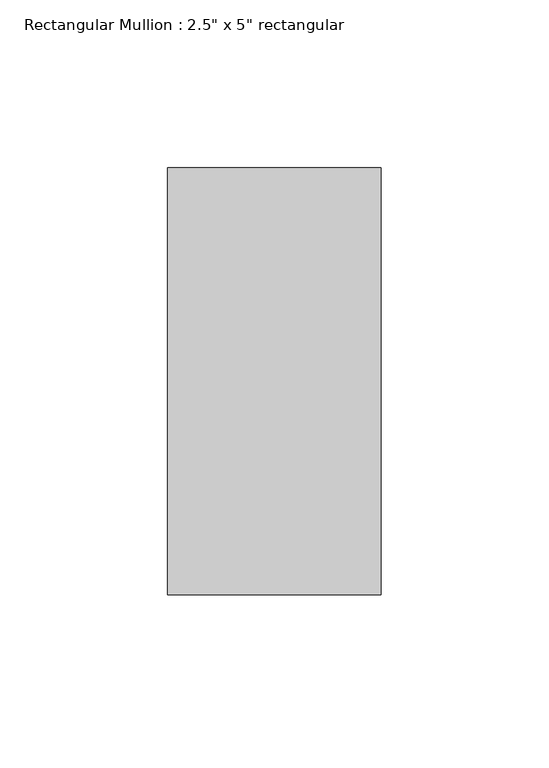
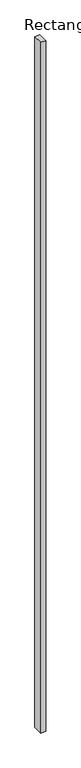
"""IFC4 building model written with IfcOpenShell, lengths in millimetres: member geometry."""

from ifc_helpers import new_model, si_unit, frame, origin, place, context, project, spatial, polyline, outline, extrude, source, transform, mapped, element, save


def member_4960e788(model_context):
    return source(origin(), model_context, "Body", "SweptSolid", [
        extrude(outline(polyline([(0.0, 63.5), (0.0, -63.5), (-63.5, -63.5), (-63.5, 63.5), (0.0, 63.5)])), frame((0.0, 0.0, -9137.65), z_axis=(0.0, 0.0, 1.0), x_axis=(1.0, 0.0, 0.0)), (0.0, 0.0, 1.0), 9137.65),
    ])


if __name__ == "__main__":
    model = new_model("IFC4")
    model_context = context("Model", 3, world=origin())
    ifc_project = project(units=[si_unit("LENGTHUNIT", "METRE", prefix="MILLI")], contexts=[model_context])
    site = spatial("IfcSite", under=ifc_project)
    building = spatial("IfcBuilding", under=site)
    placement = place(None, origin())
    member_shape = member_4960e788(model_context)
    element("IfcMember", 1, ObjectType="Rectangular Mullion : 2.5\" x 5\" rectangular", at=placement, inside=building, context=model_context, shape_type="MappedRepresentation", body=[
        mapped(member_shape, transform((0.0, 0.0, 0.0), x_axis=(1.0, 0.0, 0.0), y_axis=(0.0, 1.0, 0.0), z_axis=(0.0, 0.0, 1.0))),
    ])
    save(model, "model.ifc")

# Revit data of these elements
# Type "Rectangular Mullion : 2.5\" x 5\" rectangular"
#   built-in parameter 1007304 = 0.416667 (stored number, unit not read)
#   built-in parameter 1007301 = 0.104167 (stored number, unit not read)
#   built-in parameter 1007300 = 0.104167 (stored number, unit not read)
# Element 1 (IfcMember, "Rectangular Mullion : 2.5\" x 5\" rectangular")
#   Materials on its faces: "Aluminum"
# Materials
#   "Aluminum": class "Metal", colour RGB 247 247 247, transparency 0, Description = "Aluminum 6061", Cost = 0
